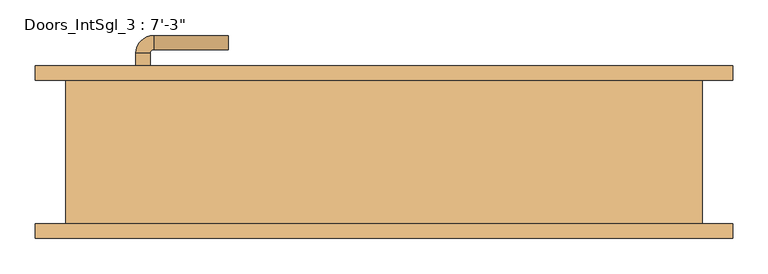
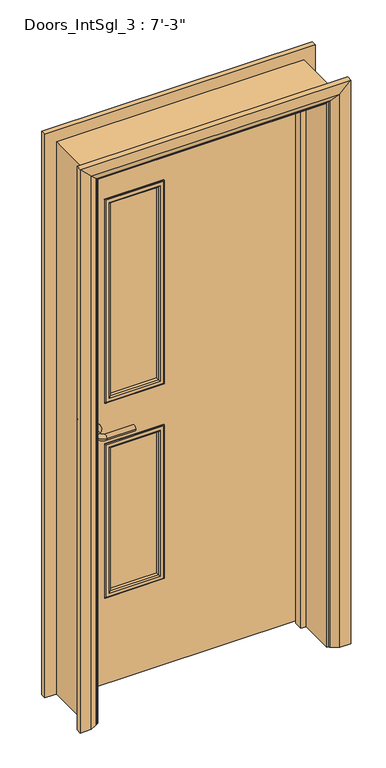
"""IFC4 building model written with IfcOpenShell, lengths in millimetres: door geometry."""

from ifc_helpers import new_model, si_unit, point, frame, frame_2d, origin, place, context, project, spatial, polyline, circle_curve, ellipse_curve, trimmed, segment, composite_curve, outline, extrude, faceted_brep, source, transform, mapped, element, save
from ifc_brep_helpers import plane_surface, cylinder_surface, revolved_surface, advanced_brep


def door_aa1d4bf3(model_context):
    return source(origin(), model_context, "Body", "SolidModel", [
        advanced_brep(
        [(-350.2, 55.6, 1000.0), (-330.2, 55.6, 1000.0), (-330.2, 25.6, 1000.0), (-350.2, 25.6, 1000.0), (-325.2, 20.6, 1000.0), (-325.2, 0.6, 1000.0), (-220.2, 0.6, 1000.0), (-220.2, 20.6, 1000.0)],
        [
            (0, 1, circle_curve(frame((-340.2, 55.6, 1000.0), z_axis=(0.0, 1.0, 0.0), x_axis=(1.0, 0.0, 0.0)), 10.0)),
            (1, 0, circle_curve(frame((-340.2, 55.6, 1000.0), z_axis=(0.0, 1.0, 0.0), x_axis=(1.0, 0.0, 0.0)), 10.0)),
            (1, 2),
            (2, 3, circle_curve(frame((-340.2, 25.6, 1000.0), z_axis=(0.0, 1.0, 0.0), x_axis=(1.0, 0.0, 0.0)), 10.0)),
            (3, 0),
            (3, 2, circle_curve(frame((-340.2, 25.6, 1000.0), z_axis=(0.0, 1.0, 0.0), x_axis=(1.0, 0.0, 0.0)), 10.0)),
            (4, 5, circle_curve(frame((-325.2, 10.6, 1000.0), z_axis=(-1.0, 0.0, 0.0), x_axis=(0.0, 1.0, 0.0)), 10.0)),
            (5, 3, circle_curve(frame((-325.2, 25.6, 1000.0), z_axis=(0.0, 0.0, -1.0), x_axis=(-1.0, 0.0, 0.0)), 25.0)),
            (2, 4, circle_curve(frame((-325.2, 25.6, 1000.0), z_axis=(0.0, 0.0, 1.0), x_axis=(-1.0, 0.0, 0.0)), 5.0)),
            (5, 4, circle_curve(frame((-325.2, 10.6, 1000.0), z_axis=(-1.0, 0.0, 0.0), x_axis=(0.0, 1.0, 0.0)), 10.0)),
            (6, 7, circle_curve(frame((-220.2, 10.6, 1000.0), z_axis=(1.0, 0.0, 0.0), x_axis=(0.0, 1.0, 0.0)), 10.0)),
            (7, 6, circle_curve(frame((-220.2, 10.6, 1000.0), z_axis=(1.0, 0.0, 0.0), x_axis=(0.0, 1.0, 0.0)), 10.0)),
            (4, 7),
            (6, 5),
        ],
        [
            plane_surface(frame((-340.2, 55.6, 1000.0), z_axis=(0.0, 1.0, 0.0), x_axis=(0.0, 0.0, 1.0))),
            cylinder_surface(frame((-340.2, 55.6, 1000.0), z_axis=(0.0, 1.0, 0.0), x_axis=(1.0, 0.0, 0.0)), 10.0),
            revolved_surface(trimmed(ellipse_curve(frame((-340.2, 25.6, 1000.0), z_axis=(0.0, -1.0, 0.0), x_axis=(1.0, 0.0, 0.0)), 10.0, 10.0), [point((-350.2, 25.6, 1000.0))], [point((-330.2, 25.6, 1000.0))], True, "CARTESIAN"), (-325.2, 25.6, 1000.0), (0.0, 0.0, -1.0)),
            revolved_surface(trimmed(ellipse_curve(frame((-340.2, 25.6, 1000.0), z_axis=(0.0, -1.0, 0.0), x_axis=(1.0, 0.0, 0.0)), 10.0, 10.0), [point((-330.2, 25.6, 1000.0))], [point((-350.2, 25.6, 1000.0))], True, "CARTESIAN"), (-325.2, 25.6, 1000.0), (0.0, 0.0, -1.0)),
            plane_surface(frame((-220.2, 10.6, 1000.0), z_axis=(1.0, 0.0, 0.0), x_axis=(0.0, 0.0, 1.0))),
            cylinder_surface(frame((-325.2, 10.6, 1000.0), z_axis=(-1.0, 0.0, 0.0), x_axis=(0.0, 1.0, 0.0)), 10.0),
        ],
        [
            (0, [[1, 2]]),
            (1, [[3, 4, 5, -2]]),
            (1, [[-5, 6, -3, -1]]),
            (2, [[7, 8, -4, 9]]),
            (3, [[10, -9, -6, -8]]),
            (4, [[11, 12]]),
            (5, [[13, -11, 14, -7]]),
            (5, [[-14, -12, -13, -10]]),
        ],
    ),
        extrude(outline(composite_curve([segment(trimmed(circle_curve(frame_2d((1000.0, -342.7)), 30.0), [point((1000.0, -372.7))], [point((1000.0, -312.7))], False, "CARTESIAN"), True, "CONTINUOUS"), segment(trimmed(circle_curve(frame_2d((1000.0, -342.7)), 30.0), [point((1000.0, -312.7))], [point((1000.0, -372.7))], False, "CARTESIAN"), True, "CONTINUOUS")], self_intersect=False)), frame((0.0, 55.6, 0.0), z_axis=(0.0, 1.0, 0.0), x_axis=(0.0, 0.0, 1.0)), (0.0, 0.0, 1.0), 8.0),
        advanced_brep(
        [(-350.2, 109.6, 1000.0), (-330.2, 109.6, 1000.0), (-350.2, 139.6, 1000.0), (-330.2, 139.6, 1000.0), (-325.2, 144.6, 1000.0), (-325.2, 164.6, 1000.0), (-220.2, 164.6, 1000.0), (-220.2, 144.6, 1000.0)],
        [
            (0, 1, circle_curve(frame((-340.2, 109.6, 1000.0), z_axis=(0.0, -1.0, 0.0), x_axis=(1.0, 0.0, 0.0)), 10.0)),
            (1, 0, circle_curve(frame((-340.2, 109.6, 1000.0), z_axis=(0.0, -1.0, 0.0), x_axis=(1.0, 0.0, 0.0)), 10.0)),
            (0, 2),
            (2, 3, circle_curve(frame((-340.2, 139.6, 1000.0), z_axis=(0.0, -1.0, 0.0), x_axis=(1.0, 0.0, 0.0)), 10.0)),
            (3, 1),
            (3, 2, circle_curve(frame((-340.2, 139.6, 1000.0), z_axis=(0.0, -1.0, 0.0), x_axis=(1.0, 0.0, 0.0)), 10.0)),
            (4, 3, circle_curve(frame((-325.2, 139.6, 1000.0), z_axis=(0.0, 0.0, 1.0), x_axis=(-1.0, 0.0, 0.0)), 5.0)),
            (2, 5, circle_curve(frame((-325.2, 139.6, 1000.0), z_axis=(0.0, 0.0, -1.0), x_axis=(-1.0, 0.0, 0.0)), 25.0)),
            (5, 4, circle_curve(frame((-325.2, 154.6, 1000.0), z_axis=(-1.0, 0.0, 0.0), x_axis=(0.0, -1.0, 0.0)), 10.0)),
            (4, 5, circle_curve(frame((-325.2, 154.6, 1000.0), z_axis=(-1.0, 0.0, 0.0), x_axis=(0.0, -1.0, 0.0)), 10.0)),
            (6, 7, circle_curve(frame((-220.2, 154.6, 1000.0), z_axis=(1.0, 0.0, 0.0), x_axis=(0.0, -1.0, 0.0)), 10.0)),
            (7, 6, circle_curve(frame((-220.2, 154.6, 1000.0), z_axis=(1.0, 0.0, 0.0), x_axis=(0.0, -1.0, 0.0)), 10.0)),
            (5, 6),
            (7, 4),
        ],
        [
            plane_surface(frame((-340.2, 109.6, 1000.0), z_axis=(0.0, -1.0, 0.0), x_axis=(0.0, 0.0, 1.0))),
            cylinder_surface(frame((-340.2, 109.6, 1000.0), z_axis=(0.0, -1.0, 0.0), x_axis=(1.0, 0.0, 0.0)), 10.0),
            revolved_surface(trimmed(ellipse_curve(frame((-340.2, 139.6, 1000.0), z_axis=(0.0, -1.0, 0.0), x_axis=(1.0, 0.0, 0.0)), 10.0, 10.0), [point((-350.2, 139.6, 1000.0))], [point((-330.2, 139.6, 1000.0))], True, "CARTESIAN"), (-325.2, 139.6, 1000.0), (0.0, 0.0, -1.0)),
            revolved_surface(trimmed(ellipse_curve(frame((-340.2, 139.6, 1000.0), z_axis=(0.0, -1.0, 0.0), x_axis=(1.0, 0.0, 0.0)), 10.0, 10.0), [point((-330.2, 139.6, 1000.0))], [point((-350.2, 139.6, 1000.0))], True, "CARTESIAN"), (-325.2, 139.6, 1000.0), (0.0, 0.0, -1.0)),
            plane_surface(frame((-220.2, 154.6, 1000.0), z_axis=(1.0, 0.0, 0.0), x_axis=(0.0, 0.0, 1.0))),
            cylinder_surface(frame((-325.2, 154.6, 1000.0), z_axis=(-1.0, 0.0, 0.0), x_axis=(0.0, -1.0, 0.0)), 10.0),
        ],
        [
            (0, [[1, 2]]),
            (1, [[-1, 3, 4, 5]]),
            (1, [[-2, -5, 6, -3]]),
            (2, [[7, -4, 8, 9]]),
            (3, [[-8, -6, -7, 10]]),
            (4, [[11, 12]]),
            (5, [[-9, 13, -12, 14]]),
            (5, [[-10, -14, -11, -13]]),
        ],
    ),
        extrude(outline(composite_curve([segment(trimmed(circle_curve(frame_2d((1000.0, -342.7)), 30.0), [point((1000.0, -372.7))], [point((1000.0, -312.7))], False, "CARTESIAN"), True, "CONTINUOUS"), segment(trimmed(circle_curve(frame_2d((1000.0, -342.7)), 30.0), [point((1000.0, -312.7))], [point((1000.0, -372.7))], False, "CARTESIAN"), True, "CONTINUOUS")], self_intersect=False)), frame((0.0, 101.6, 0.0), z_axis=(0.0, 1.0, 0.0), x_axis=(0.0, 0.0, 1.0)), (0.0, 0.0, 1.0), 8.0),
        extrude(outline(polyline([(2091.6, -415.2), (8.0, -415.2), (8.0, 415.2), (2091.6, 415.2), (2091.6, -415.2)]), holes=[polyline([(1866.6, -90.2), (1100.0, -90.2), (1100.0, -290.2), (1866.6, -290.2), (1866.6, -90.2)]), polyline([(925.0, -290.2), (925.0, -90.2), (350.0, -90.2), (350.0, -290.2), (925.0, -290.2)])]), frame((0.0, 63.6, 0.0), z_axis=(0.0, 1.0, 0.0), x_axis=(0.0, 0.0, 1.0)), (0.0, 0.0, 1.0), 38.0),
        faceted_brep([(-417.2, 101.6, 0.0), (-417.2, -101.6, 0.0), (-449.2, -101.6, 0.0), (-449.2, 101.6, 0.0), (-417.2, 101.6, 2093.6), (-417.2, -101.6, 2093.6), (-449.2, -101.6, 2125.6), (-449.2, 101.6, 2125.6), (417.2, 101.6, 0.0), (449.2, 101.6, 0.0), (449.2, -101.6, 0.0), (417.2, -101.6, 0.0), (417.2, 101.6, 2093.6), (449.2, 101.6, 2125.6), (449.2, -101.6, 2125.6), (417.2, -101.6, 2093.6)], [[[0, 1, 2, 3]], [[1, 0, 4, 5]], [[2, 1, 5, 6]], [[3, 2, 6, 7]], [[0, 3, 7, 4]], [[8, 9, 10, 11]], [[12, 13, 9, 8]], [[13, 14, 10, 9]], [[14, 15, 11, 10]], [[15, 12, 8, 11]], [[5, 4, 12, 15]], [[6, 5, 15, 14]], [[7, 6, 14, 13]], [[4, 7, 13, 12]]]),
        advanced_brep(
        [(-492.2, -121.6, 0.0), (-492.2, -101.6, 0.0), (-422.2, -101.6, 0.0), (-426.2, -107.6, 0.0), (-452.2, -121.6, 0.0), (-492.2, -121.6, 2168.6), (-492.2, -101.6, 2168.6), (-422.2, -101.6, 2098.6), (-426.2, -107.6, 2102.6), (-452.2, -121.6, 2128.6), (492.2, -121.6, 0.0), (452.2, -121.6, 0.0), (426.2, -107.6, 0.0), (422.2, -101.6, 0.0), (492.2, -101.6, 0.0), (492.2, -121.6, 2168.6), (452.2, -121.6, 2128.6), (426.2, -107.6, 2102.6), (422.2, -101.6, 2098.6), (492.2, -101.6, 2168.6)],
        [
            (0, 1),
            (1, 2),
            (2, 3, circle_curve(frame((-430.2, -100.6, 0.0), z_axis=(0.0, 0.0, -1.0), x_axis=(-1.0, 0.0, 0.0)), 8.0622577)),
            (3, 4),
            (4, 0),
            (0, 5),
            (5, 6),
            (6, 1),
            (6, 7),
            (7, 2),
            (7, 8, ellipse_curve(frame((-430.2, -100.6, 2106.6), z_axis=(-0.7071067811865475, 0.0, -0.7071067811865475), x_axis=(0.7071067811865474, 0.0, -0.7071067811865476)), 11.4017543, 8.0622577)),
            (8, 3),
            (8, 9),
            (9, 4),
            (9, 5),
            (10, 11),
            (11, 12),
            (12, 13, circle_curve(frame((430.2, -100.6, 0.0), z_axis=(0.0, 0.0, -1.0), x_axis=(1.0, 0.0, 0.0)), 8.0622577)),
            (13, 14),
            (14, 10),
            (15, 16),
            (16, 11),
            (10, 15),
            (16, 17),
            (17, 12),
            (17, 18, ellipse_curve(frame((430.2, -100.6, 2106.6), z_axis=(0.7071067811865475, 0.0, -0.7071067811865475), x_axis=(0.7071067811865474, 0.0, 0.7071067811865476)), 11.4017543, 8.0622577)),
            (18, 13),
            (18, 19),
            (19, 14),
            (19, 15),
            (5, 15),
            (19, 6),
            (18, 7),
            (17, 8),
            (16, 9),
        ],
        [
            plane_surface(frame((-422.2, -174.4010989, 0.0), z_axis=(0.0, 0.0, -1.0), x_axis=(1.0, 0.0, 0.0))),
            plane_surface(frame((-492.2, -121.6, 0.0), z_axis=(-1.0, 0.0, 0.0), x_axis=(0.0, 0.0, 1.0))),
            plane_surface(frame((-492.2, -101.6, 0.0), z_axis=(0.0, 1.0, 0.0), x_axis=(0.0, 0.0, 1.0))),
            cylinder_surface(frame((-430.2, -100.6, 0.0), z_axis=(0.0, 0.0, -1.0), x_axis=(-1.0, 0.0, 0.0)), 8.0622577),
            plane_surface(frame((-426.2, -107.6, 0.0), z_axis=(0.4740998230350183, -0.8804710999221749, 0.0), x_axis=(0.0, 0.0, 1.0))),
            plane_surface(frame((-452.2, -121.6, 0.0), z_axis=(0.0, -1.0, 0.0), x_axis=(0.0, 0.0, 1.0))),
            plane_surface(frame((422.2, -174.4010989, 0.0), z_axis=(0.0, 0.0, -1.0), x_axis=(-1.0, 0.0, 0.0))),
            plane_surface(frame((452.2, -121.6, 2128.6), z_axis=(0.0, -1.0, 0.0), x_axis=(0.0, 0.0, -1.0))),
            plane_surface(frame((426.2, -107.6, 2102.6), z_axis=(-0.4740998230350183, -0.8804710999221749, 0.0), x_axis=(0.0, 0.0, -1.0))),
            cylinder_surface(frame((430.2, -100.6, 2098.6), z_axis=(0.0, 0.0, 1.0), x_axis=(1.0, 0.0, 0.0)), 8.0622577),
            plane_surface(frame((492.2, -101.6, 2168.6), z_axis=(0.0, 1.0, 0.0), x_axis=(0.0, 0.0, -1.0))),
            plane_surface(frame((492.2, -121.6, 2168.6), z_axis=(1.0, 0.0, 0.0), x_axis=(0.0, 0.0, -1.0))),
            plane_surface(frame((-492.2, -121.6, 2168.6), z_axis=(0.0, 0.0, 1.0), x_axis=(1.0, 0.0, 0.0))),
            plane_surface(frame((-492.2, -101.6, 2168.6), z_axis=(0.0, 1.0, 0.0), x_axis=(1.0, 0.0, 0.0))),
            cylinder_surface(frame((-422.2, -100.6, 2106.6), z_axis=(-1.0, 0.0, 0.0), x_axis=(0.0, 0.0, 1.0)), 8.0622577),
            plane_surface(frame((-426.2, -107.6, 2102.6), z_axis=(0.0, -0.8804710999221749, -0.4740998230350183), x_axis=(1.0, 0.0, 0.0))),
            plane_surface(frame((-452.2, -121.6, 2128.6), z_axis=(0.0, -1.0, 0.0), x_axis=(1.0, 0.0, 0.0))),
        ],
        [
            (0, [[1, 2, 3, 4, 5]]),
            (1, [[-1, 6, 7, 8]]),
            (2, [[-2, -8, 9, 10]]),
            (3, [[-3, -10, 11, 12]]),
            (4, [[-4, -12, 13, 14]]),
            (5, [[-5, -14, 15, -6]]),
            (6, [[16, 17, 18, 19, 20]]),
            (7, [[21, 22, -16, 23]]),
            (8, [[24, 25, -17, -22]]),
            (9, [[26, 27, -18, -25]]),
            (10, [[28, 29, -19, -27]]),
            (11, [[30, -23, -20, -29]]),
            (12, [[-7, 31, -30, 32]]),
            (13, [[-9, -32, -28, 33]]),
            (14, [[-11, -33, -26, 34]]),
            (15, [[-13, -34, -24, 35]]),
            (16, [[-15, -35, -21, -31]]),
        ],
    ),
        extrude(outline(polyline([(0.0, -417.2), (0.0, -398.2), (2074.6, -398.2), (2074.6, 398.2), (0.0, 398.2), (0.0, 417.2), (2093.6, 417.2), (2093.6, -417.2), (0.0, -417.2)])), frame((0.0, 29.6, 0.0), z_axis=(0.0, 1.0, 0.0), x_axis=(0.0, 0.0, 1.0)), (0.0, 0.0, 1.0), 32.0),
        advanced_brep(
        [(492.2, 121.6, 0.0), (492.2, 101.6, 0.0), (422.2, 101.6, 0.0), (426.2, 107.6, 0.0), (452.2, 121.6, 0.0), (492.2, 121.6, 2168.6), (492.2, 101.6, 2168.6), (-492.2, 101.6, 2168.6), (-492.2, 101.6, 0.0), (-422.2, 101.6, 0.0), (-422.2, 101.6, 2098.6), (422.2, 101.6, 2098.6), (426.2, 107.6, 2102.6), (452.2, 121.6, 2128.6), (-452.2, 121.6, 2128.6), (-452.2, 121.6, 0.0), (-492.2, 121.6, 0.0), (-492.2, 121.6, 2168.6), (-426.2, 107.6, 0.0), (-426.2, 107.6, 2102.6)],
        [
            (0, 1),
            (1, 2),
            (2, 3, circle_curve(frame((430.2, 100.6, 0.0), z_axis=(0.0, 0.0, -1.0), x_axis=(1.0, 0.0, 0.0)), 8.0622577)),
            (3, 4),
            (4, 0),
            (0, 5),
            (5, 6),
            (6, 1),
            (6, 7),
            (7, 8),
            (8, 9),
            (9, 10),
            (10, 11),
            (11, 2),
            (11, 12, ellipse_curve(frame((430.2, 100.6, 2106.6), z_axis=(0.7071067811865475, 0.0, -0.7071067811865475), x_axis=(-0.7071067811865474, 0.0, -0.7071067811865476)), 11.4017543, 8.0622577)),
            (12, 3),
            (12, 13),
            (13, 4),
            (13, 14),
            (14, 15),
            (15, 16),
            (16, 17),
            (17, 5),
            (7, 17),
            (16, 8),
            (15, 18),
            (18, 9, circle_curve(frame((-430.2, 100.6, 0.0), z_axis=(0.0, 0.0, -1.0), x_axis=(-1.0, 0.0, 0.0)), 8.0622577)),
            (19, 10, ellipse_curve(frame((-430.2, 100.6, 2106.6), z_axis=(-0.7071067811865475, 0.0, -0.7071067811865475), x_axis=(-0.7071067811865474, 0.0, 0.7071067811865476)), 11.4017543, 8.0622577)),
            (18, 19),
            (14, 19),
            (19, 12),
        ],
        [
            plane_surface(frame((422.2, 101.6, 0.0), z_axis=(0.0, 0.0, -1.0), x_axis=(0.0, -1.0, 0.0))),
            plane_surface(frame((492.2, 121.6, 0.0), z_axis=(1.0, 0.0, 0.0), x_axis=(0.0, 0.0, 1.0))),
            plane_surface(frame((492.2, 101.6, 0.0), z_axis=(0.0, -1.0, 0.0), x_axis=(0.0, 0.0, 1.0))),
            cylinder_surface(frame((430.2, 100.6, 0.0), z_axis=(0.0, 0.0, -1.0), x_axis=(1.0, 0.0, 0.0)), 8.0622577),
            plane_surface(frame((426.2, 107.6, 0.0), z_axis=(-0.4740998230350126, 0.8804710999221779, 0.0), x_axis=(0.0, 0.0, 1.0))),
            plane_surface(frame((452.2, 121.6, 0.0), z_axis=(0.0, 1.0, 0.0), x_axis=(0.0, 0.0, 1.0))),
            plane_surface(frame((-492.2, 121.6, 2168.6), z_axis=(-1.0, 0.0, 0.0), x_axis=(0.0, 0.0, -1.0))),
            plane_surface(frame((-422.2, 101.6, 0.0), z_axis=(0.0, 0.0, -1.0), x_axis=(0.0, -1.0, 0.0))),
            cylinder_surface(frame((-430.2, 100.6, 2098.6), z_axis=(0.0, 0.0, 1.0), x_axis=(-1.0, 0.0, 0.0)), 8.0622577),
            plane_surface(frame((-426.2, 107.6, 2102.6), z_axis=(0.4740998230350183, 0.8804710999221749, 0.0), x_axis=(0.0, 0.0, -1.0))),
            plane_surface(frame((492.2, 121.6, 2168.6), z_axis=(0.0, 0.0, 1.0), x_axis=(-1.0, 0.0, 0.0))),
            cylinder_surface(frame((422.2, 100.6, 2106.6), z_axis=(1.0, 0.0, 0.0), x_axis=(0.0, 0.0, 1.0)), 8.0622577),
            plane_surface(frame((426.2, 107.6, 2102.6), z_axis=(0.0, 0.8804710999221763, -0.4740998230350154), x_axis=(-1.0, 0.0, 0.0))),
        ],
        [
            (0, [[1, 2, 3, 4, 5]]),
            (1, [[-1, 6, 7, 8]]),
            (2, [[-2, -8, 9, 10, 11, 12, 13, 14]]),
            (3, [[-3, -14, 15, 16]]),
            (4, [[-4, -16, 17, 18]]),
            (5, [[-5, -18, 19, 20, 21, 22, 23, -6]]),
            (6, [[24, -22, 25, -10]]),
            (7, [[-21, 26, 27, -11, -25]]),
            (8, [[28, -12, -27, 29]]),
            (9, [[30, -29, -26, -20]]),
            (10, [[-7, -23, -24, -9]]),
            (11, [[-15, -13, -28, 31]]),
            (12, [[-17, -31, -30, -19]]),
        ],
    ),
        advanced_brep(
        [(-82.2, 105.6, 1874.6), (-82.2, 101.6, 1874.6), (-82.2, 101.6, 1092.0), (-82.2, 105.6, 1092.0), (-84.2, 107.6, 1872.6), (-84.2, 107.6, 1094.0), (-102.2, 102.6, 1854.6), (-97.2, 107.6, 1859.6), (-97.2, 107.6, 1107.0), (-102.2, 102.6, 1112.0), (-102.2, 91.6, 1854.6), (-102.2, 91.6, 1112.0), (-90.2, 101.6, 1866.6), (-90.2, 91.6, 1866.6), (-90.2, 91.6, 1100.0), (-90.2, 101.6, 1100.0), (-298.2, 101.6, 1092.0), (-298.2, 105.6, 1092.0), (-296.2, 107.6, 1094.0), (-283.2, 107.6, 1107.0), (-278.2, 102.6, 1112.0), (-278.2, 91.6, 1112.0), (-290.2, 91.6, 1100.0), (-290.2, 101.6, 1100.0), (-298.2, 101.6, 1874.6), (-298.2, 105.6, 1874.6), (-296.2, 107.6, 1872.6), (-283.2, 107.6, 1859.6), (-278.2, 102.6, 1854.6), (-278.2, 91.6, 1854.6), (-290.2, 91.6, 1866.6), (-290.2, 101.6, 1866.6)],
        [
            (0, 1),
            (1, 2),
            (2, 3),
            (3, 0),
            (4, 0, ellipse_curve(frame((-84.2, 105.6, 1872.6), z_axis=(0.7071067811865475, 0.0, -0.7071067811865475), x_axis=(0.7071067811865474, 0.0, 0.7071067811865476)), 2.8284271, 2.0)),
            (3, 5, ellipse_curve(frame((-84.2, 105.6, 1094.0), z_axis=(0.7071067811865475, 0.0, 0.7071067811865475), x_axis=(-0.7071067811865474, 0.0, 0.7071067811865476)), 2.8284271, 2.0)),
            (5, 4),
            (6, 7, ellipse_curve(frame((-97.2, 102.6, 1859.6), z_axis=(0.7071067811865475, 0.0, -0.7071067811865475), x_axis=(0.7071067811865474, 0.0, 0.7071067811865476)), 7.0710678, 5.0)),
            (7, 8),
            (8, 9, ellipse_curve(frame((-97.2, 102.6, 1107.0), z_axis=(0.7071067811865475, 0.0, 0.7071067811865475), x_axis=(-0.7071067811865474, 0.0, 0.7071067811865476)), 7.0710678, 5.0)),
            (9, 6),
            (10, 6),
            (9, 11),
            (11, 10),
            (12, 13),
            (13, 14),
            (14, 15),
            (15, 12),
            (2, 16),
            (16, 17),
            (17, 3),
            (17, 18, ellipse_curve(frame((-296.2, 105.6, 1094.0), z_axis=(0.7071067811865475, 0.0, -0.7071067811865475), x_axis=(0.7071067811865476, 0.0, 0.7071067811865474)), 2.8284271, 2.0)),
            (18, 5),
            (8, 19),
            (19, 20, ellipse_curve(frame((-283.2, 102.6, 1107.0), z_axis=(0.7071067811865475, 0.0, -0.7071067811865475), x_axis=(0.7071067811865476, 0.0, 0.7071067811865474)), 7.0710678, 5.0)),
            (20, 9),
            (20, 21),
            (21, 11),
            (14, 22),
            (22, 23),
            (23, 15),
            (16, 24),
            (24, 25),
            (25, 17),
            (25, 26, ellipse_curve(frame((-296.2, 105.6, 1872.6), z_axis=(-0.7071067811865475, 0.0, -0.7071067811865475), x_axis=(0.7071067811865474, 0.0, -0.7071067811865476)), 2.8284271, 2.0)),
            (26, 18),
            (19, 27),
            (27, 28, ellipse_curve(frame((-283.2, 102.6, 1859.6), z_axis=(-0.7071067811865475, 0.0, -0.7071067811865475), x_axis=(0.7071067811865474, 0.0, -0.7071067811865476)), 7.0710678, 5.0)),
            (28, 20),
            (28, 29),
            (29, 21),
            (22, 30),
            (30, 31),
            (31, 23),
            (24, 1),
            (0, 25),
            (4, 26),
            (7, 27),
            (6, 28),
            (10, 29),
            (13, 30),
            (12, 31),
        ],
        [
            plane_surface(frame((-82.2, 101.6, 1874.6), z_axis=(1.0, 0.0, 0.0), x_axis=(0.0, 0.0, -1.0))),
            cylinder_surface(frame((-84.2, 105.6, 1866.6), z_axis=(0.0, 0.0, 1.0), x_axis=(1.0, 0.0, 0.0)), 2.0),
            cylinder_surface(frame((-97.2, 102.6, 1866.6), z_axis=(0.0, 0.0, 1.0), x_axis=(1.0, 0.0, 0.0)), 5.0),
            plane_surface(frame((-102.2, 102.6, 1854.6), z_axis=(-1.0, 0.0, 0.0), x_axis=(0.0, 0.0, -1.0))),
            plane_surface(frame((-90.2, 91.6, 1866.6), z_axis=(1.0, 0.0, 0.0), x_axis=(0.0, 0.0, -1.0))),
            plane_surface(frame((-82.2, 101.6, 1092.0), z_axis=(0.0, 0.0, -1.0), x_axis=(-1.0, 0.0, 0.0))),
            cylinder_surface(frame((-90.2, 105.6, 1094.0), z_axis=(1.0, 0.0, 0.0), x_axis=(0.0, 0.0, -1.0)), 2.0),
            cylinder_surface(frame((-90.2, 102.6, 1107.0), z_axis=(1.0, 0.0, 0.0), x_axis=(0.0, 0.0, -1.0)), 5.0),
            plane_surface(frame((-102.2, 102.6, 1112.0), z_axis=(0.0, 0.0, 1.0), x_axis=(-1.0, 0.0, 0.0))),
            plane_surface(frame((-90.2, 91.6, 1100.0), z_axis=(0.0, 0.0, -1.0), x_axis=(-1.0, 0.0, 0.0))),
            plane_surface(frame((-298.2, 101.6, 1092.0), z_axis=(-1.0, 0.0, 0.0), x_axis=(0.0, 0.0, 1.0))),
            cylinder_surface(frame((-296.2, 105.6, 1100.0), z_axis=(0.0, 0.0, -1.0), x_axis=(-1.0, 0.0, 0.0)), 2.0),
            cylinder_surface(frame((-283.2, 102.6, 1100.0), z_axis=(0.0, 0.0, -1.0), x_axis=(-1.0, 0.0, 0.0)), 5.0),
            plane_surface(frame((-278.2, 102.6, 1112.0), z_axis=(1.0, 0.0, 0.0), x_axis=(0.0, 0.0, 1.0))),
            plane_surface(frame((-290.2, 91.6, 1100.0), z_axis=(-1.0, 0.0, 0.0), x_axis=(0.0, 0.0, 1.0))),
            plane_surface(frame((-298.2, 101.6, 1874.6), z_axis=(0.0, 0.0, 1.0), x_axis=(1.0, 0.0, 0.0))),
            cylinder_surface(frame((-290.2, 105.6, 1872.6), z_axis=(-1.0, 0.0, 0.0), x_axis=(0.0, 0.0, 1.0)), 2.0),
            plane_surface(frame((-296.2, 107.6, 1872.6), z_axis=(0.0, 1.0, 0.0), x_axis=(1.0, 0.0, 0.0))),
            cylinder_surface(frame((-290.2, 102.6, 1859.6), z_axis=(-1.0, 0.0, 0.0), x_axis=(0.0, 0.0, 1.0)), 5.0),
            plane_surface(frame((-278.2, 102.6, 1854.6), z_axis=(0.0, 0.0, -1.0), x_axis=(1.0, 0.0, 0.0))),
            plane_surface(frame((-278.2, 91.6, 1854.6), z_axis=(0.0, -1.0, 0.0), x_axis=(1.0, 0.0, 0.0))),
            plane_surface(frame((-290.2, 91.6, 1866.6), z_axis=(0.0, 0.0, 1.0), x_axis=(1.0, 0.0, 0.0))),
            plane_surface(frame((-290.2, 101.6, 1866.6), z_axis=(0.0, -1.0, 0.0), x_axis=(1.0, 0.0, 0.0))),
        ],
        [
            (0, [[1, 2, 3, 4]]),
            (1, [[5, -4, 6, 7]]),
            (2, [[8, 9, 10, 11]]),
            (3, [[12, -11, 13, 14]]),
            (4, [[15, 16, 17, 18]]),
            (5, [[-3, 19, 20, 21]]),
            (6, [[-6, -21, 22, 23]]),
            (7, [[-10, 24, 25, 26]]),
            (8, [[-13, -26, 27, 28]]),
            (9, [[-17, 29, 30, 31]]),
            (10, [[-20, 32, 33, 34]]),
            (11, [[-22, -34, 35, 36]]),
            (12, [[-25, 37, 38, 39]]),
            (13, [[-27, -39, 40, 41]]),
            (14, [[-30, 42, 43, 44]]),
            (15, [[-33, 45, -1, 46]]),
            (16, [[-35, -46, -5, 47]]),
            (17, [[-23, -36, -47, -7], [48, -37, -24, -9]]),
            (18, [[-38, -48, -8, 49]]),
            (19, [[-40, -49, -12, 50]]),
            (20, [[51, -42, -29, -16], [-28, -41, -50, -14]]),
            (21, [[-43, -51, -15, 52]]),
            (22, [[-45, -32, -19, -2], [-31, -44, -52, -18]]),
        ],
    ),
        advanced_brep(
        [(-90.2, 73.6, 1866.6), (-90.2, 63.6, 1866.6), (-90.2, 63.6, 1100.0), (-90.2, 73.6, 1100.0), (-102.2, 62.6, 1854.6), (-102.2, 73.6, 1854.6), (-102.2, 73.6, 1112.0), (-102.2, 62.6, 1112.0), (-97.2, 57.6, 1859.6), (-97.2, 57.6, 1107.0), (-82.2, 59.6, 1874.6), (-84.2, 57.6, 1872.6), (-84.2, 57.6, 1094.0), (-82.2, 59.6, 1092.0), (-82.2, 63.6, 1874.6), (-82.2, 63.6, 1092.0), (-290.2, 63.6, 1100.0), (-290.2, 73.6, 1100.0), (-278.2, 73.6, 1112.0), (-278.2, 62.6, 1112.0), (-283.2, 57.6, 1107.0), (-296.2, 57.6, 1094.0), (-298.2, 59.6, 1092.0), (-298.2, 63.6, 1092.0), (-290.2, 63.6, 1866.6), (-290.2, 73.6, 1866.6), (-278.2, 73.6, 1854.6), (-278.2, 62.6, 1854.6), (-283.2, 57.6, 1859.6), (-296.2, 57.6, 1872.6), (-298.2, 59.6, 1874.6), (-298.2, 63.6, 1874.6)],
        [
            (0, 1),
            (1, 2),
            (2, 3),
            (3, 0),
            (4, 5),
            (5, 6),
            (6, 7),
            (7, 4),
            (8, 4, ellipse_curve(frame((-97.2, 62.6, 1859.6), z_axis=(0.7071067811865475, 0.0, -0.7071067811865475), x_axis=(0.7071067811865474, 0.0, 0.7071067811865476)), 7.0710678, 5.0)),
            (7, 9, ellipse_curve(frame((-97.2, 62.6, 1107.0), z_axis=(0.7071067811865475, 0.0, 0.7071067811865475), x_axis=(-0.7071067811865474, 0.0, 0.7071067811865476)), 7.0710678, 5.0)),
            (9, 8),
            (10, 11, ellipse_curve(frame((-84.2, 59.6, 1872.6), z_axis=(0.7071067811865475, 0.0, -0.7071067811865475), x_axis=(0.7071067811865474, 0.0, 0.7071067811865476)), 2.8284271, 2.0)),
            (11, 12),
            (12, 13, ellipse_curve(frame((-84.2, 59.6, 1094.0), z_axis=(0.7071067811865475, 0.0, 0.7071067811865475), x_axis=(-0.7071067811865474, 0.0, 0.7071067811865476)), 2.8284271, 2.0)),
            (13, 10),
            (14, 10),
            (13, 15),
            (15, 14),
            (2, 16),
            (16, 17),
            (17, 3),
            (6, 18),
            (18, 19),
            (19, 7),
            (19, 20, ellipse_curve(frame((-283.2, 62.6, 1107.0), z_axis=(0.7071067811865475, 0.0, -0.7071067811865475), x_axis=(0.7071067811865476, 0.0, 0.7071067811865474)), 7.0710678, 5.0)),
            (20, 9),
            (12, 21),
            (21, 22, ellipse_curve(frame((-296.2, 59.6, 1094.0), z_axis=(0.7071067811865475, 0.0, -0.7071067811865475), x_axis=(0.7071067811865476, 0.0, 0.7071067811865474)), 2.8284271, 2.0)),
            (22, 13),
            (22, 23),
            (23, 15),
            (16, 24),
            (24, 25),
            (25, 17),
            (18, 26),
            (26, 27),
            (27, 19),
            (27, 28, ellipse_curve(frame((-283.2, 62.6, 1859.6), z_axis=(-0.7071067811865475, 0.0, -0.7071067811865475), x_axis=(0.7071067811865474, 0.0, -0.7071067811865476)), 7.0710678, 5.0)),
            (28, 20),
            (21, 29),
            (29, 30, ellipse_curve(frame((-296.2, 59.6, 1872.6), z_axis=(-0.7071067811865475, 0.0, -0.7071067811865475), x_axis=(0.7071067811865474, 0.0, -0.7071067811865476)), 2.8284271, 2.0)),
            (30, 22),
            (30, 31),
            (31, 23),
            (31, 14),
            (1, 24),
            (0, 25),
            (5, 26),
            (4, 27),
            (8, 28),
            (11, 29),
            (10, 30),
        ],
        [
            plane_surface(frame((-90.2, 63.6, 1866.6), z_axis=(1.0, 0.0, 0.0), x_axis=(0.0, 0.0, -1.0))),
            plane_surface(frame((-102.2, 73.6, 1854.6), z_axis=(-1.0, 0.0, 0.0), x_axis=(0.0, 0.0, -1.0))),
            cylinder_surface(frame((-97.2, 62.6, 1866.6), z_axis=(0.0, 0.0, 1.0), x_axis=(1.0, 0.0, 0.0)), 5.0),
            cylinder_surface(frame((-84.2, 59.6, 1866.6), z_axis=(0.0, 0.0, 1.0), x_axis=(1.0, 0.0, 0.0)), 2.0),
            plane_surface(frame((-82.2, 59.6, 1874.6), z_axis=(1.0, 0.0, 0.0), x_axis=(0.0, 0.0, -1.0))),
            plane_surface(frame((-90.2, 63.6, 1100.0), z_axis=(0.0, 0.0, -1.0), x_axis=(-1.0, 0.0, 0.0))),
            plane_surface(frame((-102.2, 73.6, 1112.0), z_axis=(0.0, 0.0, 1.0), x_axis=(-1.0, 0.0, 0.0))),
            cylinder_surface(frame((-90.2, 62.6, 1107.0), z_axis=(1.0, 0.0, 0.0), x_axis=(0.0, 0.0, -1.0)), 5.0),
            cylinder_surface(frame((-90.2, 59.6, 1094.0), z_axis=(1.0, 0.0, 0.0), x_axis=(0.0, 0.0, -1.0)), 2.0),
            plane_surface(frame((-82.2, 59.6, 1092.0), z_axis=(0.0, 0.0, -1.0), x_axis=(-1.0, 0.0, 0.0))),
            plane_surface(frame((-290.2, 63.6, 1100.0), z_axis=(-1.0, 0.0, 0.0), x_axis=(0.0, 0.0, 1.0))),
            plane_surface(frame((-278.2, 73.6, 1112.0), z_axis=(1.0, 0.0, 0.0), x_axis=(0.0, 0.0, 1.0))),
            cylinder_surface(frame((-283.2, 62.6, 1100.0), z_axis=(0.0, 0.0, -1.0), x_axis=(-1.0, 0.0, 0.0)), 5.0),
            cylinder_surface(frame((-296.2, 59.6, 1100.0), z_axis=(0.0, 0.0, -1.0), x_axis=(-1.0, 0.0, 0.0)), 2.0),
            plane_surface(frame((-298.2, 59.6, 1092.0), z_axis=(-1.0, 0.0, 0.0), x_axis=(0.0, 0.0, 1.0))),
            plane_surface(frame((-298.2, 63.6, 1874.6), z_axis=(0.0, 1.0, 0.0), x_axis=(1.0, 0.0, 0.0))),
            plane_surface(frame((-290.2, 63.6, 1866.6), z_axis=(0.0, 0.0, 1.0), x_axis=(1.0, 0.0, 0.0))),
            plane_surface(frame((-290.2, 73.6, 1866.6), z_axis=(0.0, 1.0, 0.0), x_axis=(1.0, 0.0, 0.0))),
            plane_surface(frame((-278.2, 73.6, 1854.6), z_axis=(0.0, 0.0, -1.0), x_axis=(1.0, 0.0, 0.0))),
            cylinder_surface(frame((-290.2, 62.6, 1859.6), z_axis=(-1.0, 0.0, 0.0), x_axis=(0.0, 0.0, 1.0)), 5.0),
            plane_surface(frame((-283.2, 57.6, 1859.6), z_axis=(0.0, -1.0, 0.0), x_axis=(1.0, 0.0, 0.0))),
            cylinder_surface(frame((-290.2, 59.6, 1872.6), z_axis=(-1.0, 0.0, 0.0), x_axis=(0.0, 0.0, 1.0)), 2.0),
            plane_surface(frame((-298.2, 59.6, 1874.6), z_axis=(0.0, 0.0, 1.0), x_axis=(1.0, 0.0, 0.0))),
        ],
        [
            (0, [[1, 2, 3, 4]]),
            (1, [[5, 6, 7, 8]]),
            (2, [[9, -8, 10, 11]]),
            (3, [[12, 13, 14, 15]]),
            (4, [[16, -15, 17, 18]]),
            (5, [[-3, 19, 20, 21]]),
            (6, [[-7, 22, 23, 24]]),
            (7, [[-10, -24, 25, 26]]),
            (8, [[-14, 27, 28, 29]]),
            (9, [[-17, -29, 30, 31]]),
            (10, [[-20, 32, 33, 34]]),
            (11, [[-23, 35, 36, 37]]),
            (12, [[-25, -37, 38, 39]]),
            (13, [[-28, 40, 41, 42]]),
            (14, [[-30, -42, 43, 44]]),
            (15, [[-31, -44, 45, -18], [46, -32, -19, -2]]),
            (16, [[-33, -46, -1, 47]]),
            (17, [[-21, -34, -47, -4], [48, -35, -22, -6]]),
            (18, [[-36, -48, -5, 49]]),
            (19, [[-38, -49, -9, 50]]),
            (20, [[51, -40, -27, -13], [-26, -39, -50, -11]]),
            (21, [[-41, -51, -12, 52]]),
            (22, [[-43, -52, -16, -45]]),
        ],
    ),
        extrude(outline(polyline([(-290.2, 91.6), (-90.2, 91.6), (-90.2, 73.6), (-290.2, 73.6), (-290.2, 91.6)])), frame((0.0, 0.0, 1100.0), z_axis=(0.0, 0.0, 1.0), x_axis=(1.0, 0.0, 0.0)), (0.0, 0.0, 1.0), 766.6),
        extrude(outline(polyline([(-290.2, 91.6), (-90.2, 91.6), (-90.2, 73.6), (-290.2, 73.6), (-290.2, 91.6)])), frame((0.0, 0.0, 350.0), z_axis=(0.0, 0.0, 1.0), x_axis=(1.0, 0.0, 0.0)), (0.0, 0.0, 1.0), 575.0),
        advanced_brep(
        [(-290.2, 91.6, 925.0), (-290.2, 101.6, 925.0), (-290.2, 101.6, 350.0), (-290.2, 91.6, 350.0), (-278.2, 102.6, 913.0), (-278.2, 91.6, 913.0), (-278.2, 91.6, 362.0), (-278.2, 102.6, 362.0), (-283.2, 107.6, 918.0), (-283.2, 107.6, 357.0), (-298.2, 105.6, 933.0), (-296.2, 107.6, 931.0), (-296.2, 107.6, 344.0), (-298.2, 105.6, 342.0), (-298.2, 101.6, 933.0), (-298.2, 101.6, 342.0), (-90.2, 101.6, 350.0), (-90.2, 91.6, 350.0), (-102.2, 91.6, 362.0), (-102.2, 102.6, 362.0), (-97.2, 107.6, 357.0), (-84.2, 107.6, 344.0), (-82.2, 105.6, 342.0), (-82.2, 101.6, 342.0), (-90.2, 101.6, 925.0), (-90.2, 91.6, 925.0), (-102.2, 91.6, 913.0), (-102.2, 102.6, 913.0), (-97.2, 107.6, 918.0), (-84.2, 107.6, 931.0), (-82.2, 105.6, 933.0), (-82.2, 101.6, 933.0)],
        [
            (0, 1),
            (1, 2),
            (2, 3),
            (3, 0),
            (4, 5),
            (5, 6),
            (6, 7),
            (7, 4),
            (8, 4, ellipse_curve(frame((-283.2, 102.6, 918.0), z_axis=(-0.7071067811865475, 0.0, -0.7071067811865475), x_axis=(-0.7071067811865474, 0.0, 0.7071067811865476)), 7.0710678, 5.0)),
            (7, 9, ellipse_curve(frame((-283.2, 102.6, 357.0), z_axis=(-0.7071067811865475, 0.0, 0.7071067811865475), x_axis=(0.7071067811865474, 0.0, 0.7071067811865476)), 7.0710678, 5.0)),
            (9, 8),
            (10, 11, ellipse_curve(frame((-296.2, 105.6, 931.0), z_axis=(-0.7071067811865475, 0.0, -0.7071067811865475), x_axis=(-0.7071067811865474, 0.0, 0.7071067811865476)), 2.8284271, 2.0)),
            (11, 12),
            (12, 13, ellipse_curve(frame((-296.2, 105.6, 344.0), z_axis=(-0.7071067811865475, 0.0, 0.7071067811865475), x_axis=(0.7071067811865474, 0.0, 0.7071067811865476)), 2.8284271, 2.0)),
            (13, 10),
            (14, 10),
            (13, 15),
            (15, 14),
            (2, 16),
            (16, 17),
            (17, 3),
            (6, 18),
            (18, 19),
            (19, 7),
            (19, 20, ellipse_curve(frame((-97.2, 102.6, 357.0), z_axis=(-0.7071067811865475, 0.0, -0.7071067811865475), x_axis=(-0.7071067811865476, 0.0, 0.7071067811865474)), 7.0710678, 5.0)),
            (20, 9),
            (12, 21),
            (21, 22, ellipse_curve(frame((-84.2, 105.6, 344.0), z_axis=(-0.7071067811865475, 0.0, -0.7071067811865475), x_axis=(-0.7071067811865476, 0.0, 0.7071067811865474)), 2.8284271, 2.0)),
            (22, 13),
            (22, 23),
            (23, 15),
            (16, 24),
            (24, 25),
            (25, 17),
            (18, 26),
            (26, 27),
            (27, 19),
            (27, 28, ellipse_curve(frame((-97.2, 102.6, 918.0), z_axis=(0.7071067811865475, 0.0, -0.7071067811865475), x_axis=(-0.7071067811865474, 0.0, -0.7071067811865476)), 7.0710678, 5.0)),
            (28, 20),
            (21, 29),
            (29, 30, ellipse_curve(frame((-84.2, 105.6, 931.0), z_axis=(0.7071067811865475, 0.0, -0.7071067811865475), x_axis=(-0.7071067811865474, 0.0, -0.7071067811865476)), 2.8284271, 2.0)),
            (30, 22),
            (30, 31),
            (31, 23),
            (31, 14),
            (1, 24),
            (0, 25),
            (5, 26),
            (4, 27),
            (8, 28),
            (11, 29),
            (10, 30),
        ],
        [
            plane_surface(frame((-290.2, 101.6, 925.0), z_axis=(-1.0, 0.0, 0.0), x_axis=(0.0, 0.0, -1.0))),
            plane_surface(frame((-278.2, 91.6, 913.0), z_axis=(1.0, 0.0, 0.0), x_axis=(0.0, 0.0, -1.0))),
            cylinder_surface(frame((-283.2, 102.6, 925.0), z_axis=(0.0, 0.0, 1.0), x_axis=(-1.0, 0.0, 0.0)), 5.0),
            cylinder_surface(frame((-296.2, 105.6, 925.0), z_axis=(0.0, 0.0, 1.0), x_axis=(-1.0, 0.0, 0.0)), 2.0),
            plane_surface(frame((-298.2, 105.6, 933.0), z_axis=(-1.0, 0.0, 0.0), x_axis=(0.0, 0.0, -1.0))),
            plane_surface(frame((-290.2, 101.6, 350.0), z_axis=(0.0, 0.0, -1.0), x_axis=(1.0, 0.0, 0.0))),
            plane_surface(frame((-278.2, 91.6, 362.0), z_axis=(0.0, 0.0, 1.0), x_axis=(1.0, 0.0, 0.0))),
            cylinder_surface(frame((-290.2, 102.6, 357.0), z_axis=(-1.0, 0.0, 0.0), x_axis=(0.0, 0.0, -1.0)), 5.0),
            cylinder_surface(frame((-290.2, 105.6, 344.0), z_axis=(-1.0, 0.0, 0.0), x_axis=(0.0, 0.0, -1.0)), 2.0),
            plane_surface(frame((-298.2, 105.6, 342.0), z_axis=(0.0, 0.0, -1.0), x_axis=(1.0, 0.0, 0.0))),
            plane_surface(frame((-90.2, 101.6, 350.0), z_axis=(1.0, 0.0, 0.0), x_axis=(0.0, 0.0, 1.0))),
            plane_surface(frame((-102.2, 91.6, 362.0), z_axis=(-1.0, 0.0, 0.0), x_axis=(0.0, 0.0, 1.0))),
            cylinder_surface(frame((-97.2, 102.6, 350.0), z_axis=(0.0, 0.0, -1.0), x_axis=(1.0, 0.0, 0.0)), 5.0),
            cylinder_surface(frame((-84.2, 105.6, 350.0), z_axis=(0.0, 0.0, -1.0), x_axis=(1.0, 0.0, 0.0)), 2.0),
            plane_surface(frame((-82.2, 105.6, 342.0), z_axis=(1.0, 0.0, 0.0), x_axis=(0.0, 0.0, 1.0))),
            plane_surface(frame((-82.2, 101.6, 933.0), z_axis=(0.0, -1.0, 0.0), x_axis=(-1.0, 0.0, 0.0))),
            plane_surface(frame((-90.2, 101.6, 925.0), z_axis=(0.0, 0.0, 1.0), x_axis=(-1.0, 0.0, 0.0))),
            plane_surface(frame((-90.2, 91.6, 925.0), z_axis=(0.0, -1.0, 0.0), x_axis=(-1.0, 0.0, 0.0))),
            plane_surface(frame((-102.2, 91.6, 913.0), z_axis=(0.0, 0.0, -1.0), x_axis=(-1.0, 0.0, 0.0))),
            cylinder_surface(frame((-90.2, 102.6, 918.0), z_axis=(1.0, 0.0, 0.0), x_axis=(0.0, 0.0, 1.0)), 5.0),
            plane_surface(frame((-97.2, 107.6, 918.0), z_axis=(0.0, 1.0, 0.0), x_axis=(-1.0, 0.0, 0.0))),
            cylinder_surface(frame((-90.2, 105.6, 931.0), z_axis=(1.0, 0.0, 0.0), x_axis=(0.0, 0.0, 1.0)), 2.0),
            plane_surface(frame((-82.2, 105.6, 933.0), z_axis=(0.0, 0.0, 1.0), x_axis=(-1.0, 0.0, 0.0))),
        ],
        [
            (0, [[1, 2, 3, 4]]),
            (1, [[5, 6, 7, 8]]),
            (2, [[9, -8, 10, 11]]),
            (3, [[12, 13, 14, 15]]),
            (4, [[16, -15, 17, 18]]),
            (5, [[-3, 19, 20, 21]]),
            (6, [[-7, 22, 23, 24]]),
            (7, [[-10, -24, 25, 26]]),
            (8, [[-14, 27, 28, 29]]),
            (9, [[-17, -29, 30, 31]]),
            (10, [[-20, 32, 33, 34]]),
            (11, [[-23, 35, 36, 37]]),
            (12, [[-25, -37, 38, 39]]),
            (13, [[-28, 40, 41, 42]]),
            (14, [[-30, -42, 43, 44]]),
            (15, [[-31, -44, 45, -18], [46, -32, -19, -2]]),
            (16, [[-33, -46, -1, 47]]),
            (17, [[-21, -34, -47, -4], [48, -35, -22, -6]]),
            (18, [[-36, -48, -5, 49]]),
            (19, [[-38, -49, -9, 50]]),
            (20, [[51, -40, -27, -13], [-26, -39, -50, -11]]),
            (21, [[-41, -51, -12, 52]]),
            (22, [[-43, -52, -16, -45]]),
        ],
    ),
        advanced_brep(
        [(-90.2, 73.6, 925.0), (-90.2, 63.6, 925.0), (-90.2, 63.6, 350.0), (-90.2, 73.6, 350.0), (-102.2, 62.6, 913.0), (-102.2, 73.6, 913.0), (-102.2, 73.6, 362.0), (-102.2, 62.6, 362.0), (-97.2, 57.6, 918.0), (-97.2, 57.6, 357.0), (-82.2, 59.6, 933.0), (-84.2, 57.6, 931.0), (-84.2, 57.6, 344.0), (-82.2, 59.6, 342.0), (-82.2, 63.6, 933.0), (-82.2, 63.6, 342.0), (-290.2, 63.6, 350.0), (-290.2, 73.6, 350.0), (-278.2, 73.6, 362.0), (-278.2, 62.6, 362.0), (-283.2, 57.6, 357.0), (-296.2, 57.6, 344.0), (-298.2, 59.6, 342.0), (-298.2, 63.6, 342.0), (-290.2, 63.6, 925.0), (-290.2, 73.6, 925.0), (-278.2, 73.6, 913.0), (-278.2, 62.6, 913.0), (-283.2, 57.6, 918.0), (-296.2, 57.6, 931.0), (-298.2, 59.6, 933.0), (-298.2, 63.6, 933.0)],
        [
            (0, 1),
            (1, 2),
            (2, 3),
            (3, 0),
            (4, 5),
            (5, 6),
            (6, 7),
            (7, 4),
            (8, 4, ellipse_curve(frame((-97.2, 62.6, 918.0), z_axis=(0.7071067811865475, 0.0, -0.7071067811865475), x_axis=(0.7071067811865474, 0.0, 0.7071067811865476)), 7.0710678, 5.0)),
            (7, 9, ellipse_curve(frame((-97.2, 62.6, 357.0), z_axis=(0.7071067811865475, 0.0, 0.7071067811865475), x_axis=(-0.7071067811865474, 0.0, 0.7071067811865476)), 7.0710678, 5.0)),
            (9, 8),
            (10, 11, ellipse_curve(frame((-84.2, 59.6, 931.0), z_axis=(0.7071067811865475, 0.0, -0.7071067811865475), x_axis=(0.7071067811865474, 0.0, 0.7071067811865476)), 2.8284271, 2.0)),
            (11, 12),
            (12, 13, ellipse_curve(frame((-84.2, 59.6, 344.0), z_axis=(0.7071067811865475, 0.0, 0.7071067811865475), x_axis=(-0.7071067811865474, 0.0, 0.7071067811865476)), 2.8284271, 2.0)),
            (13, 10),
            (14, 10),
            (13, 15),
            (15, 14),
            (2, 16),
            (16, 17),
            (17, 3),
            (6, 18),
            (18, 19),
            (19, 7),
            (19, 20, ellipse_curve(frame((-283.2, 62.6, 357.0), z_axis=(0.7071067811865475, 0.0, -0.7071067811865475), x_axis=(0.7071067811865476, 0.0, 0.7071067811865474)), 7.0710678, 5.0)),
            (20, 9),
            (12, 21),
            (21, 22, ellipse_curve(frame((-296.2, 59.6, 344.0), z_axis=(0.7071067811865475, 0.0, -0.7071067811865475), x_axis=(0.7071067811865476, 0.0, 0.7071067811865474)), 2.8284271, 2.0)),
            (22, 13),
            (22, 23),
            (23, 15),
            (16, 24),
            (24, 25),
            (25, 17),
            (18, 26),
            (26, 27),
            (27, 19),
            (27, 28, ellipse_curve(frame((-283.2, 62.6, 918.0), z_axis=(-0.7071067811865475, 0.0, -0.7071067811865475), x_axis=(0.7071067811865474, 0.0, -0.7071067811865476)), 7.0710678, 5.0)),
            (28, 20),
            (21, 29),
            (29, 30, ellipse_curve(frame((-296.2, 59.6, 931.0), z_axis=(-0.7071067811865475, 0.0, -0.7071067811865475), x_axis=(0.7071067811865474, 0.0, -0.7071067811865476)), 2.8284271, 2.0)),
            (30, 22),
            (30, 31),
            (31, 23),
            (31, 14),
            (1, 24),
            (0, 25),
            (5, 26),
            (4, 27),
            (8, 28),
            (11, 29),
            (10, 30),
        ],
        [
            plane_surface(frame((-90.2, 63.6, 925.0), z_axis=(1.0, 0.0, 0.0), x_axis=(0.0, 0.0, -1.0))),
            plane_surface(frame((-102.2, 73.6, 913.0), z_axis=(-1.0, 0.0, 0.0), x_axis=(0.0, 0.0, -1.0))),
            cylinder_surface(frame((-97.2, 62.6, 925.0), z_axis=(0.0, 0.0, 1.0), x_axis=(1.0, 0.0, 0.0)), 5.0),
            cylinder_surface(frame((-84.2, 59.6, 925.0), z_axis=(0.0, 0.0, 1.0), x_axis=(1.0, 0.0, 0.0)), 2.0),
            plane_surface(frame((-82.2, 59.6, 933.0), z_axis=(1.0, 0.0, 0.0), x_axis=(0.0, 0.0, -1.0))),
            plane_surface(frame((-90.2, 63.6, 350.0), z_axis=(0.0, 0.0, -1.0), x_axis=(-1.0, 0.0, 0.0))),
            plane_surface(frame((-102.2, 73.6, 362.0), z_axis=(0.0, 0.0, 1.0), x_axis=(-1.0, 0.0, 0.0))),
            cylinder_surface(frame((-90.2, 62.6, 357.0), z_axis=(1.0, 0.0, 0.0), x_axis=(0.0, 0.0, -1.0)), 5.0),
            cylinder_surface(frame((-90.2, 59.6, 344.0), z_axis=(1.0, 0.0, 0.0), x_axis=(0.0, 0.0, -1.0)), 2.0),
            plane_surface(frame((-82.2, 59.6, 342.0), z_axis=(0.0, 0.0, -1.0), x_axis=(-1.0, 0.0, 0.0))),
            plane_surface(frame((-290.2, 63.6, 350.0), z_axis=(-1.0, 0.0, 0.0), x_axis=(0.0, 0.0, 1.0))),
            plane_surface(frame((-278.2, 73.6, 362.0), z_axis=(1.0, 0.0, 0.0), x_axis=(0.0, 0.0, 1.0))),
            cylinder_surface(frame((-283.2, 62.6, 350.0), z_axis=(0.0, 0.0, -1.0), x_axis=(-1.0, 0.0, 0.0)), 5.0),
            cylinder_surface(frame((-296.2, 59.6, 350.0), z_axis=(0.0, 0.0, -1.0), x_axis=(-1.0, 0.0, 0.0)), 2.0),
            plane_surface(frame((-298.2, 59.6, 342.0), z_axis=(-1.0, 0.0, 0.0), x_axis=(0.0, 0.0, 1.0))),
            plane_surface(frame((-298.2, 63.6, 933.0), z_axis=(0.0, 1.0, 0.0), x_axis=(1.0, 0.0, 0.0))),
            plane_surface(frame((-290.2, 63.6, 925.0), z_axis=(0.0, 0.0, 1.0), x_axis=(1.0, 0.0, 0.0))),
            plane_surface(frame((-290.2, 73.6, 925.0), z_axis=(0.0, 1.0, 0.0), x_axis=(1.0, 0.0, 0.0))),
            plane_surface(frame((-278.2, 73.6, 913.0), z_axis=(0.0, 0.0, -1.0), x_axis=(1.0, 0.0, 0.0))),
            cylinder_surface(frame((-290.2, 62.6, 918.0), z_axis=(-1.0, 0.0, 0.0), x_axis=(0.0, 0.0, 1.0)), 5.0),
            plane_surface(frame((-283.2, 57.6, 918.0), z_axis=(0.0, -1.0, 0.0), x_axis=(1.0, 0.0, 0.0))),
            cylinder_surface(frame((-290.2, 59.6, 931.0), z_axis=(-1.0, 0.0, 0.0), x_axis=(0.0, 0.0, 1.0)), 2.0),
            plane_surface(frame((-298.2, 59.6, 933.0), z_axis=(0.0, 0.0, 1.0), x_axis=(1.0, 0.0, 0.0))),
        ],
        [
            (0, [[1, 2, 3, 4]]),
            (1, [[5, 6, 7, 8]]),
            (2, [[9, -8, 10, 11]]),
            (3, [[12, 13, 14, 15]]),
            (4, [[16, -15, 17, 18]]),
            (5, [[-3, 19, 20, 21]]),
            (6, [[-7, 22, 23, 24]]),
            (7, [[-10, -24, 25, 26]]),
            (8, [[-14, 27, 28, 29]]),
            (9, [[-17, -29, 30, 31]]),
            (10, [[-20, 32, 33, 34]]),
            (11, [[-23, 35, 36, 37]]),
            (12, [[-25, -37, 38, 39]]),
            (13, [[-28, 40, 41, 42]]),
            (14, [[-30, -42, 43, 44]]),
            (15, [[-31, -44, 45, -18], [46, -32, -19, -2]]),
            (16, [[-33, -46, -1, 47]]),
            (17, [[-21, -34, -47, -4], [48, -35, -22, -6]]),
            (18, [[-36, -48, -5, 49]]),
            (19, [[-38, -49, -9, 50]]),
            (20, [[51, -40, -27, -13], [-26, -39, -50, -11]]),
            (21, [[-41, -51, -12, 52]]),
            (22, [[-43, -52, -16, -45]]),
        ],
    ),
    ])


if __name__ == "__main__":
    model = new_model("IFC4")
    model_context = context("Model", 3, world=origin())
    ifc_project = project(units=[si_unit("LENGTHUNIT", "METRE", prefix="MILLI")], contexts=[model_context])
    site = spatial("IfcSite", under=ifc_project)
    building = spatial("IfcBuilding", under=site)
    placement = place(None, origin())
    door_shape = door_aa1d4bf3(model_context)
    element("IfcDoor", 1, ObjectType="Doors_IntSgl_3 : 7'-3\"", at=placement, inside=building, context=model_context, shape_type="MappedRepresentation", body=[
        mapped(door_shape, transform((0.0, 0.0, 0.0), x_axis=(1.0, 0.0, 0.0), y_axis=(0.0, 1.0, 0.0), z_axis=(0.0, 0.0, 1.0))),
    ])
    save(model, "model.ifc")

# Revit data of these elements
# Type "Doors_IntSgl_3 : 7'-3\""
#   Type Mark = "14"
#   Type Comments = "Internal Single"
#   Operation = "SingleSwingRight"
#   Construction Type Id = "SGL"
#   Manufacturer = "Revit"
#   Keynote = "L20"
#   Description = "Internal Single Door"
#   Analytic Construction = "Large single-glazed windows"
#   Visual Light Transmittance = 0.9
#   VisionPanel Width = 0' - 7.87402"
#   UnderCut = 0' - 0.31496"
#   Tolerance = 0' - 0.07874"
#   Structural Tolerance = 0' - 0.31496"
#   StopDepth = 0' - 1.25984"
#   Stop Thickness = 0' - 0.74803"
#   Stile Top of Lock Rail = 3' - 7.30709"
#   Stile Top Rail = 0' - 8.85827"
#   Stile Shutting = 0' - 4.92126"
#   Stile Lock Rail = 0' - 6.88976"
#   Stile Bottom Rail = 1' - 1.77953"
#   Solar Heat Gain Coefficient = 0.86
#   Rough Width = 3' - 0"
#   Rough Height = 7' - 0"
#   Heat Transfer Coefficient (U) = 0.979472 BTU/(h·ft²·°F)
#   Handle Z Distance = 3' - 3.37008"
#   Handle X Distance = 0' - 2.95276"
#   Frame Thickness = 0' - 1.25984"
#   Door Panel Width = 2' - 8.69291"
#   Door Panel Thickness = 0' - 1.49606"
#   Door Panel Offset = 0' - 0"
#   Height = 7' - 0"
#   Width = 3' - 0"
#   Door Panel Height = 6' - 10.0315"
#   Architrave Setback = 0' - 0.19685"
#   Vis - Ironmongery = yes
#   Define Thermal Properties by = 1
#   Material Ironmongery = Door - Handle
#   Material Glass = Door - Glazing
#   Material Frame = Door - Frame/Mullion
#   Material Door = Door - Panel
#   Material Beading = Door - Panel
#   Material Architrave = Door - Architrave
#   Function = (empty or 0)
#   Wall Closure = (empty or 0)
# Element 1 (IfcDoor, "Doors_IntSgl_3 : 7'-3\"")
#   Materials on its faces: "Door - Panel", "Door - Architrave", "Door - Handle", "Door - Frame/Mullion", "Door - Glazing"
# Materials
#   "Door - Handle": colour RGB 246 240 166, transparency 0
#   "Door - Glazing": colour RGB 0 0 255, transparency 0.75
#   "Door - Frame/Mullion": class "Wood", colour RGB 212 179 113, transparency 0
#   "Door - Panel": class "Wood", colour RGB 210 159 95, transparency 0, Cost = 0
#   "Door - Architrave": class "Wood", colour RGB 212 179 113, transparency 0
